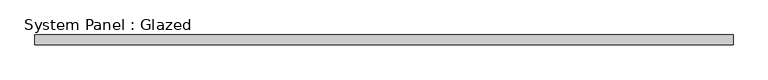
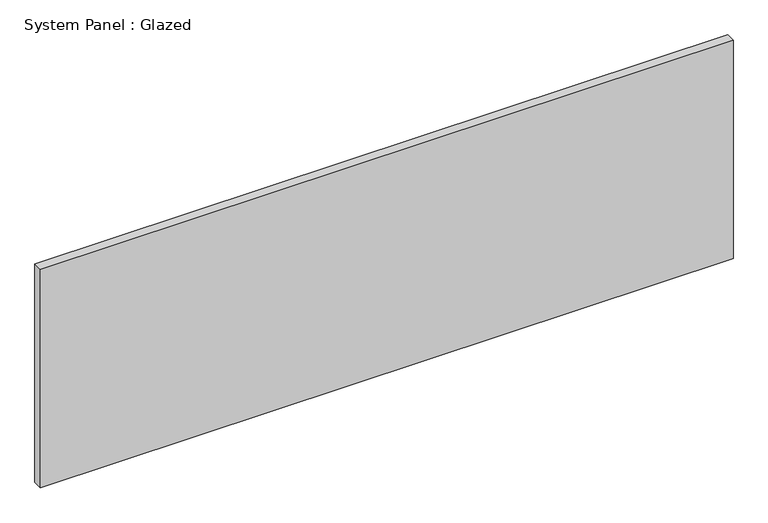
"""IFC4 building model written with IfcOpenShell, lengths in millimetres: plate geometry, System Panel : Glazed."""

from ifc_helpers import new_model, si_unit, origin, origin_with_axes, place, context, project, spatial, polyline, outline, extrude, source, transform, mapped, element, save


def system_panel_glazed_63189bcd(model_context):
    return source(origin(), model_context, "Body", "SweptSolid", [
        extrude(outline(polyline([(914.4, 19.05), (-914.4, 19.05), (-914.4, 44.45), (914.4, 44.45), (914.4, 19.05)])), origin_with_axes(), (0.0, 0.0, 1.0), 609.6),
    ])


if __name__ == "__main__":
    model = new_model("IFC4")
    model_context = context("Model", 3, world=origin())
    ifc_project = project(units=[si_unit("LENGTHUNIT", "METRE", prefix="MILLI")], contexts=[model_context])
    site = spatial("IfcSite", under=ifc_project)
    building = spatial("IfcBuilding", under=site)
    placement = place(None, origin())
    system_panel_glazed_shape = system_panel_glazed_63189bcd(model_context)
    element("IfcPlate", 1, ObjectType="System Panel : Glazed", at=placement, inside=building, context=model_context, shape_type="MappedRepresentation", body=[
        mapped(system_panel_glazed_shape, transform((0.0, 0.0, 0.0), x_axis=(1.0, 0.0, 0.0), y_axis=(0.0, 1.0, 0.0), z_axis=(0.0, 0.0, 1.0))),
    ])
    save(model, "model.ifc")

# Revit data of these elements
# Type "System Panel : Glazed"
#   Construction Type Id = "GSP4R"
#   Analytic Construction = "1/8 in Pilkington single glazing"
#   Visual Light Transmittance = 0.9
#   Solar Heat Gain Coefficient = 0.86
#   Heat Transfer Coefficient (U) = 1.18115 BTU/(h·ft²·°F)
# Element 1 (IfcPlate, "System Panel : Glazed")
#   Materials on its faces: "Glass"
# Materials
#   "Glass": class "Glass", colour RGB 0 128 192, transparency 0.75, Description = "Soda Lime Glass", Cost = 0
